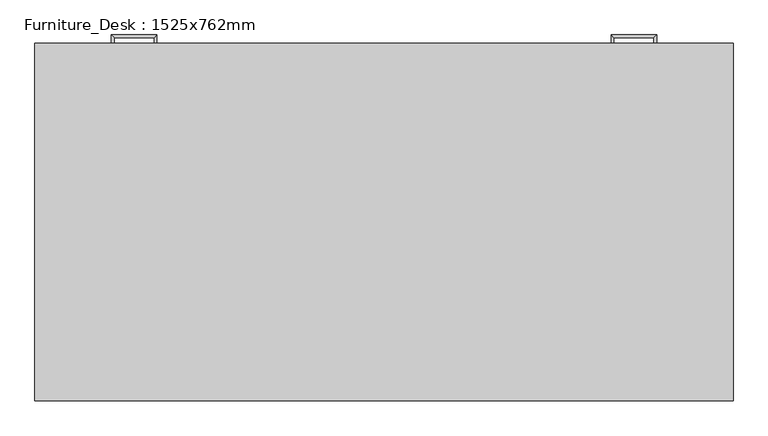
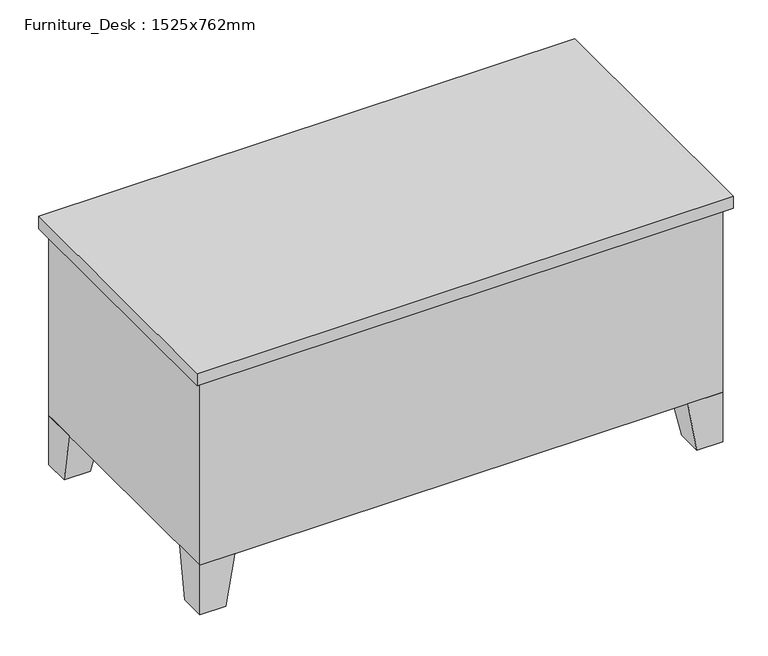
"""IFC4 building model written with IfcOpenShell, lengths in millimetres: furniture geometry, Furniture_Desk : 1525x762mm."""

from ifc_helpers import new_model, si_unit, frame, origin, place, context, project, spatial, polyline, outline, extrude, faceted_brep, source, transform, mapped, element, save


def furniture_desk_1525x762mm_aed207d5(model_context):
    return source(origin(), model_context, "Body", "SolidModel", [
        extrude(outline(polyline([(1505.95, 762.0), (1137.65, 762.0), (1137.65, 774.7), (1505.95, 774.7), (1505.95, 762.0)])), frame((0.0, 0.0, 603.25), z_axis=(0.0, 0.0, 1.0), x_axis=(1.0, 0.0, 0.0)), (0.0, 0.0, 1.0), 101.6),
        extrude(outline(polyline([(1505.95, 762.0), (1137.65, 762.0), (1137.65, 774.7), (1505.95, 774.7), (1505.95, 762.0)])), frame((0.0, 0.0, 171.05), z_axis=(0.0, 0.0, 1.0), x_axis=(1.0, 0.0, 0.0)), (0.0, 0.0, 1.0), 413.15),
        extrude(outline(polyline([(387.35, 762.0), (19.05, 762.0), (19.05, 774.7), (387.35, 774.7), (387.35, 762.0)])), frame((0.0, 0.0, 602.85), z_axis=(0.0, 0.0, 1.0), x_axis=(1.0, 0.0, 0.0)), (0.0, 0.0, 1.0), 102.0),
        extrude(outline(polyline([(387.35, 762.0), (19.05, 762.0), (19.05, 774.7), (387.35, 774.7), (387.35, 762.0)])), frame((0.0, 0.0, 171.05), z_axis=(0.0, 0.0, 1.0), x_axis=(1.0, 0.0, 0.0)), (0.0, 0.0, 1.0), 171.45),
        extrude(outline(polyline([(387.35, 762.0), (19.05, 762.0), (19.05, 774.7), (387.35, 774.7), (387.35, 762.0)])), frame((0.0, 0.0, 482.2), z_axis=(0.0, 0.0, 1.0), x_axis=(1.0, 0.0, 0.0)), (0.0, 0.0, 1.0), 101.6),
        extrude(outline(polyline([(387.35, 762.0), (19.05, 762.0), (19.05, 774.7), (387.35, 774.7), (387.35, 762.0)])), frame((0.0, 0.0, 361.55), z_axis=(0.0, 0.0, 1.0), x_axis=(1.0, 0.0, 0.0)), (0.0, 0.0, 1.0), 101.6),
        faceted_brep([(1423.4, 762.0, 152.0), (1423.4, 660.4, 152.0), (1525.0, 660.4, 152.0), (1525.0, 762.0, 152.0), (1448.8, 762.0, 0.0), (1525.0, 762.0, 0.0), (1525.0, 685.8, 0.0), (1448.8, 685.8, 0.0)], [[[0, 1, 2, 3]], [[4, 5, 6, 7]], [[4, 7, 1, 0]], [[7, 6, 2, 1]], [[6, 5, 3, 2]], [[5, 4, 0, 3]]]),
        faceted_brep([(1423.4, 0.0, 152.0), (1525.0, 0.0, 152.0), (1525.0, 101.6, 152.0), (1423.4, 101.6, 152.0), (1448.8, 0.0, 0.0), (1448.8, 76.2, 0.0), (1525.0, 76.2, 0.0), (1525.0, 0.0, 0.0)], [[[0, 1, 2, 3]], [[4, 5, 6, 7]], [[4, 7, 1, 0]], [[7, 6, 2, 1]], [[6, 5, 3, 2]], [[5, 4, 0, 3]]]),
        faceted_brep([(101.6, 0.0, 152.0), (101.6, 101.6, 152.0), (0.0, 101.6, 152.0), (0.0, 0.0, 152.0), (76.2, 0.0, 0.0), (0.0, 0.0, 0.0), (0.0, 76.2, 0.0), (76.2, 76.2, 0.0)], [[[0, 1, 2, 3]], [[4, 5, 6, 7]], [[4, 7, 1, 0]], [[7, 6, 2, 1]], [[6, 5, 3, 2]], [[5, 4, 0, 3]]]),
        faceted_brep([(101.6, 762.0, 152.0), (0.0, 762.0, 152.0), (0.0, 660.4, 152.0), (101.6, 660.4, 152.0), (76.2, 762.0, 0.0), (76.2, 685.8, 0.0), (0.0, 685.8, 0.0), (0.0, 762.0, 0.0)], [[[0, 1, 2, 3]], [[4, 5, 6, 7]], [[4, 7, 1, 0]], [[7, 6, 2, 1]], [[6, 5, 3, 2]], [[5, 4, 0, 3]]]),
        extrude(outline(polyline([(1544.05, 781.05), (1544.05, -19.05), (-19.05, -19.05), (-19.05, 781.05), (1544.05, 781.05)])), frame((0.0, 0.0, 723.9), z_axis=(0.0, 0.0, 1.0), x_axis=(1.0, 0.0, 0.0)), (0.0, 0.0, 1.0), 38.1),
        extrude(outline(polyline([(406.4, 762.0), (406.4, 50.8), (1118.6, 50.8), (1118.6, 762.0), (1525.0, 762.0), (1525.0, 0.0), (0.0, 0.0), (0.0, 762.0), (406.4, 762.0)])), frame((0.0, 0.0, 152.0), z_axis=(0.0, 0.0, 1.0), x_axis=(1.0, 0.0, 0.0)), (0.0, 0.0, 1.0), 571.9),
        faceted_brep([(1366.25, 774.7, 546.1), (1366.25, 774.7, 533.4), (1372.6, 774.7, 533.4), (1372.6, 774.7, 546.1), (1366.25, 793.75, 546.1), (1366.25, 793.75, 533.4), (1372.6, 800.1, 533.4), (1372.6, 800.1, 546.1), (1277.35, 793.75, 546.1), (1277.35, 793.75, 533.4), (1271.0, 800.1, 533.4), (1271.0, 800.1, 546.1), (1277.35, 774.7, 546.1), (1271.0, 774.7, 546.1), (1271.0, 774.7, 533.4), (1277.35, 774.7, 533.4)], [[[0, 1, 2, 3]], [[1, 0, 4, 5]], [[2, 1, 5, 6]], [[3, 2, 6, 7]], [[0, 3, 7, 4]], [[5, 4, 8, 9]], [[6, 5, 9, 10]], [[7, 6, 10, 11]], [[4, 7, 11, 8]], [[12, 13, 14, 15]], [[9, 8, 12, 15]], [[10, 9, 15, 14]], [[11, 10, 14, 13]], [[8, 11, 13, 12]]]),
        faceted_brep([(1366.25, 774.7, 666.75), (1366.25, 774.7, 654.05), (1372.6, 774.7, 654.05), (1372.6, 774.7, 666.75), (1366.25, 793.75, 666.75), (1366.25, 793.75, 654.05), (1372.6, 800.1, 654.05), (1372.6, 800.1, 666.75), (1277.35, 793.75, 666.75), (1277.35, 793.75, 654.05), (1271.0, 800.1, 654.05), (1271.0, 800.1, 666.75), (1277.35, 774.7, 666.75), (1271.0, 774.7, 666.75), (1271.0, 774.7, 654.05), (1277.35, 774.7, 654.05)], [[[0, 1, 2, 3]], [[1, 0, 4, 5]], [[2, 1, 5, 6]], [[3, 2, 6, 7]], [[0, 3, 7, 4]], [[5, 4, 8, 9]], [[6, 5, 9, 10]], [[7, 6, 10, 11]], [[4, 7, 11, 8]], [[12, 13, 14, 15]], [[9, 8, 12, 15]], [[10, 9, 15, 14]], [[11, 10, 14, 13]], [[8, 11, 13, 12]]]),
        faceted_brep([(158.75, 774.7, 304.8), (152.4, 774.7, 304.8), (152.4, 774.7, 292.1), (158.75, 774.7, 292.1), (158.75, 793.75, 304.8), (152.4, 800.1, 304.8), (152.4, 800.1, 292.1), (158.75, 793.75, 292.1), (247.65, 793.75, 304.8), (254.0, 800.1, 304.8), (254.0, 800.1, 292.1), (247.65, 793.75, 292.1), (247.65, 774.7, 304.8), (247.65, 774.7, 292.1), (254.0, 774.7, 292.1), (254.0, 774.7, 304.8)], [[[0, 1, 2, 3]], [[1, 0, 4, 5]], [[2, 1, 5, 6]], [[3, 2, 6, 7]], [[0, 3, 7, 4]], [[5, 4, 8, 9]], [[6, 5, 9, 10]], [[7, 6, 10, 11]], [[4, 7, 11, 8]], [[12, 13, 14, 15]], [[9, 8, 12, 15]], [[10, 9, 15, 14]], [[11, 10, 14, 13]], [[8, 11, 13, 12]]]),
        faceted_brep([(158.75, 774.7, 425.45), (152.4, 774.7, 425.45), (152.4, 774.7, 412.75), (158.75, 774.7, 412.75), (158.75, 793.75, 425.45), (152.4, 800.1, 425.45), (152.4, 800.1, 412.75), (158.75, 793.75, 412.75), (247.65, 793.75, 425.45), (254.0, 800.1, 425.45), (254.0, 800.1, 412.75), (247.65, 793.75, 412.75), (247.65, 774.7, 425.45), (247.65, 774.7, 412.75), (254.0, 774.7, 412.75), (254.0, 774.7, 425.45)], [[[0, 1, 2, 3]], [[1, 0, 4, 5]], [[2, 1, 5, 6]], [[3, 2, 6, 7]], [[0, 3, 7, 4]], [[5, 4, 8, 9]], [[6, 5, 9, 10]], [[7, 6, 10, 11]], [[4, 7, 11, 8]], [[12, 13, 14, 15]], [[9, 8, 12, 15]], [[10, 9, 15, 14]], [[11, 10, 14, 13]], [[8, 11, 13, 12]]]),
        faceted_brep([(158.75, 774.7, 546.1), (152.4, 774.7, 546.1), (152.4, 774.7, 533.4), (158.75, 774.7, 533.4), (158.75, 793.75, 546.1), (152.4, 800.1, 546.1), (152.4, 800.1, 533.4), (158.75, 793.75, 533.4), (247.65, 793.75, 546.1), (254.0, 800.1, 546.1), (254.0, 800.1, 533.4), (247.65, 793.75, 533.4), (247.65, 774.7, 546.1), (247.65, 774.7, 533.4), (254.0, 774.7, 533.4), (254.0, 774.7, 546.1)], [[[0, 1, 2, 3]], [[1, 0, 4, 5]], [[2, 1, 5, 6]], [[3, 2, 6, 7]], [[0, 3, 7, 4]], [[5, 4, 8, 9]], [[6, 5, 9, 10]], [[7, 6, 10, 11]], [[4, 7, 11, 8]], [[12, 13, 14, 15]], [[9, 8, 12, 15]], [[10, 9, 15, 14]], [[11, 10, 14, 13]], [[8, 11, 13, 12]]]),
        faceted_brep([(158.75, 774.7, 666.75), (152.4, 774.7, 666.75), (152.4, 774.7, 654.05), (158.75, 774.7, 654.05), (158.75, 793.75, 666.75), (152.4, 800.1, 666.75), (152.4, 800.1, 654.05), (158.75, 793.75, 654.05), (247.65, 793.75, 666.75), (254.0, 800.1, 666.75), (254.0, 800.1, 654.05), (247.65, 793.75, 654.05), (247.65, 774.7, 666.75), (247.65, 774.7, 654.05), (254.0, 774.7, 654.05), (254.0, 774.7, 666.75)], [[[0, 1, 2, 3]], [[1, 0, 4, 5]], [[2, 1, 5, 6]], [[3, 2, 6, 7]], [[0, 3, 7, 4]], [[5, 4, 8, 9]], [[6, 5, 9, 10]], [[7, 6, 10, 11]], [[4, 7, 11, 8]], [[12, 13, 14, 15]], [[9, 8, 12, 15]], [[10, 9, 15, 14]], [[11, 10, 14, 13]], [[8, 11, 13, 12]]]),
    ])


if __name__ == "__main__":
    model = new_model("IFC4")
    model_context = context("Model", 3, world=origin())
    ifc_project = project(units=[si_unit("LENGTHUNIT", "METRE", prefix="MILLI")], contexts=[model_context])
    site = spatial("IfcSite", under=ifc_project)
    building = spatial("IfcBuilding", under=site)
    placement = place(None, origin())
    furniture_desk_1525x762mm_shape = furniture_desk_1525x762mm_aed207d5(model_context)
    element("IfcFurniture", 1, ObjectType="Furniture_Desk : 1525x762mm", at=placement, inside=building, context=model_context, shape_type="MappedRepresentation", body=[
        mapped(furniture_desk_1525x762mm_shape, transform((0.0, 0.0, 0.0), x_axis=(1.0, 0.0, 0.0), y_axis=(0.0, 1.0, 0.0), z_axis=(0.0, 0.0, 1.0))),
    ])
    save(model, "model.ifc")

# Revit data of these elements
# Type "Furniture_Desk : 1525x762mm"
#   Keynote = "N"
#   Width = 1525 mm
#   Leg Height = 152 mm
#   Height = 762 mm
#   Depth = 762 mm
#   Top Material = Cherry
#   Handle/Leg Material = Steel, Chrome Plated
#   Body Material = Laminate, Ivory, Matte
#   Default Elevation = 0
#   Assembly Code = ""
# Element 1 (IfcFurniture, "Furniture_Desk : 1525x762mm")
#   Materials on its faces: "Steel, Chrome Plated", "Laminate, Ivory, Matte", "Cherry"
# Materials
#   "Cherry": class "Wood", colour RGB 226 177 128, transparency 0, Description = "Prunus Serotina", Cost = 0
#   "Steel, Chrome Plated": class "Metal", colour RGB 216 216 216, transparency 0, Description = "Chromiuim plated steel", Cost = 0
#   "Laminate, Ivory, Matte": class "Plastic", colour RGB 247 247 239, transparency 0, Description = "Plastic Laminate - Ivory, Matte", Cost = 0
